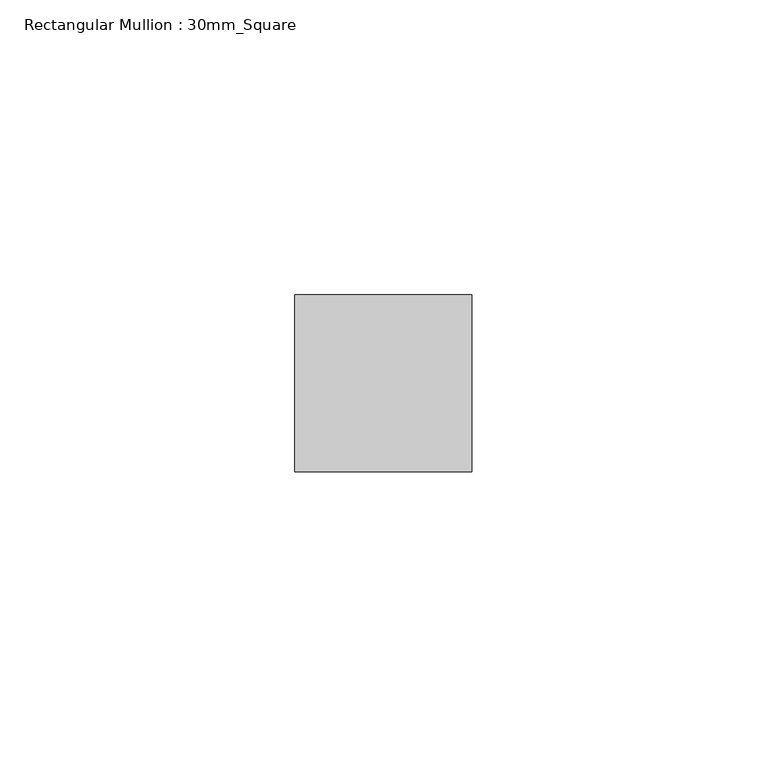
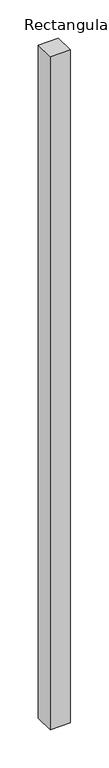
"""IFC4 building model written with IfcOpenShell, lengths in millimetres: member geometry, Rectangular Mullion : 30mm_Square."""

from ifc_helpers import new_model, si_unit, frame, origin, place, context, project, spatial, polyline, outline, extrude, source, transform, mapped, element, save


def rectangular_mullion_30mm_square_508dbaa4(model_context):
    return source(origin(), model_context, "Body", "SweptSolid", [
        extrude(outline(polyline([(0.0, 15.0), (0.0, -15.0), (-30.0, -15.0), (-30.0, 15.0), (0.0, 15.0)])), frame((0.0, 0.0, -1067.1518548), z_axis=(0.0, 0.0, 1.0), x_axis=(1.0, 0.0, 0.0)), (0.0, 0.0, 1.0), 1067.1518548),
    ])


if __name__ == "__main__":
    model = new_model("IFC4")
    model_context = context("Model", 3, world=origin())
    ifc_project = project(units=[si_unit("LENGTHUNIT", "METRE", prefix="MILLI")], contexts=[model_context])
    site = spatial("IfcSite", under=ifc_project)
    building = spatial("IfcBuilding", under=site)
    placement = place(None, origin())
    rectangular_mullion_30mm_square_shape = rectangular_mullion_30mm_square_508dbaa4(model_context)
    element("IfcMember", 1, ObjectType="Rectangular Mullion : 30mm_Square", at=placement, inside=building, context=model_context, shape_type="MappedRepresentation", body=[
        mapped(rectangular_mullion_30mm_square_shape, transform((0.0, 0.0, 0.0), x_axis=(1.0, 0.0, 0.0), y_axis=(0.0, 1.0, 0.0), z_axis=(0.0, 0.0, 1.0))),
    ])
    save(model, "model.ifc")

# Revit data of these elements
# Type "Rectangular Mullion : 30mm_Square"
#   Keynote = "H11"
#   built-in parameter 1007304 = 0.0984252 (stored number, unit not read)
#   built-in parameter 1007301 = 0.0492126 (stored number, unit not read)
#   built-in parameter 1007300 = 0.0492126 (stored number, unit not read)
# Element 1 (IfcMember, "Rectangular Mullion : 30mm_Square")
#   Materials on its faces: "Aluminium"
# Materials
#   "Aluminium": class "Metal", colour RGB 247 247 247, transparency 0, Description = "Aluminium 6061", Cost = 0
